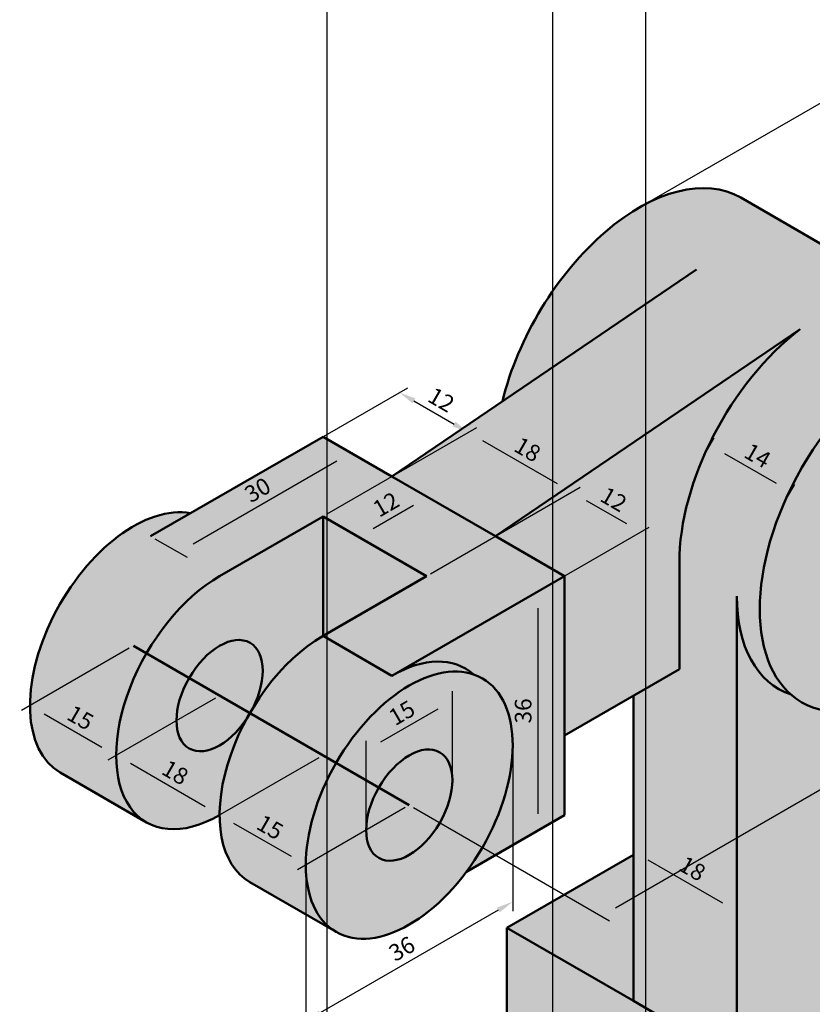
# Model space of a CAD drawing. Units: millimetres. Extents: x 1466 to 1886, y 5011 to 5605.
# Tile 3 of 4: x 1677 to 1796, y 5146 to 5295. Entities that reach past the tile are written whole.
import ezdxf

# ---------------------------------------------------------------- set-up
doc = ezdxf.new("R2010")
doc.units = ezdxf.units.MM
for name, color, linetype, lineweight in [('M-DIMS', 2, 'Continuous', 25), ('M-HATC', 252, 'Continuous', 18), ('M-OUTL', 7, 'Continuous', 50)]:
    doc.layers.add(name, color=color, linetype=linetype, lineweight=lineweight)
doc.styles.get("Standard").update_dxf_attribs({"font": 'arial.ttf'})
doc.dimstyles.new('ISO-25', dxfattribs={"dimtxt": 2.5, "dimasz": 2.5, "dimexe": 1.25, "dimexo": 0.625, "dimtad": 1, "dimtxsty": 'Standard', "dimcen": 2.5, "dimadec": 0, "dimazin": 0, "dimtfac": 1, "dimtmove": 0, "dimatfit": 3, "dimfxl": 1, "dimarcsym": 0})

# ---------------------------------------------------------------- blocks, each defined once
blk = doc.blocks.new('*D1')
at = {"layer": 'Defpoints', "color": 0, "transparency": 16777216}
for p in [(1828.098835256636, 5162.955036981139), (1834.164568784784, 5159.452984095829), (1784.797565067414, 5137.955036981139)]:
    blk.add_point(p, dxfattribs=at)
at = {"layer": 'M-DIMS', "color": 0, "lineweight": -2, "transparency": 16777216}
for p, q in [((1828.723835256636, 5162.594193062894), (1835.414568784784, 5158.731296259342)), ((1793.028362105023, 5135.702984095829), (1831.999505275323, 5158.202984095829)), ((1785.422565067414, 5137.594193062894), (1792.113298595562, 5133.731296259342))]:
    blk.add_line(p, q, dxfattribs=at)
at = {"layer": 'M-DIMS', "color": 0, "transparency": 16777216}
for points in [[(1831.79117194199, 5158.563828014073), (1832.207838608656, 5157.842140177587), (1834.164568784784, 5159.452984095829)], [(1792.82002877169, 5136.063828014073), (1793.236695438357, 5135.342140177587), (1790.863298595562, 5134.45298409583)]]:
    blk.add_solid(points, dxfattribs=at)
at = {"layer": 'M-DIMS', "color": 0, "transparency": 16777216, "insert": (1811.563217455521, 5148.599672917828), "char_height": 2.5, "attachment_point": 5, "rotation": 30.000000000000025}
blk.add_mtext('50', dxfattribs=at)
blk = doc.blocks.new('*D3')
at = {"layer": 'Defpoints', "color": 0, "transparency": 16777216}
for p in [(1770.344853030102, 5217.610759795876), (1738.032193263054, 5210.955036981139), (1748.424498108467, 5204.955036981139)]:
    blk.add_point(p, dxfattribs=at)
at = {"layer": 'M-DIMS', "color": 0, "lineweight": -2, "transparency": 16777216}
for p, q in [((1738.657193263054, 5211.315880899382), (1761.202548184689, 5224.332447632363)), ((1762.11761169415, 5222.360759795876), (1768.179789520641, 5218.860759795877)), ((1749.049498108467, 5205.315880899382), (1771.594853030102, 5218.332447632363))]:
    blk.add_line(p, q, dxfattribs=at)
at = {"layer": 'M-DIMS', "color": 0, "transparency": 16777216}
for points in [[(1762.325945027483, 5222.72160371412), (1761.909278360817, 5221.999915877631), (1759.952548184689, 5223.610759795876)], [(1768.388122853975, 5219.22160371412), (1767.971456187307, 5218.499915877632), (1770.344853030102, 5217.610759795876)]]:
    blk.add_solid(points, dxfattribs=at)
at = {"layer": 'M-DIMS', "color": 0, "transparency": 16777216, "insert": (1766.088758588296, 5222.238987980856), "char_height": 2.5, "attachment_point": 5, "rotation": 330}
blk.add_mtext('12', dxfattribs=at)
blk = doc.blocks.new('*D4')
at = {"layer": 'Defpoints', "color": 0, "transparency": 16777216}
for p in [(1744.364090916567, 5232.610759795876), (1722.443735994934, 5219.955036981137), (1738.032193263055, 5210.955036981139)]:
    blk.add_point(p, dxfattribs=at)
at = {"layer": 'M-DIMS', "color": 0, "lineweight": -2, "transparency": 16777216}
for p, q in [((1723.068735994934, 5220.315880899381), (1745.614090916567, 5233.332447632363)), ((1757.787484675226, 5224.860759795877), (1746.529154426028, 5231.360759795876)), ((1738.657193263054, 5211.315880899382), (1761.202548184687, 5224.332447632364))]:
    blk.add_line(p, q, dxfattribs=at)
at = {"layer": 'M-DIMS', "color": 0, "transparency": 16777216}
for points in [[(1746.737487759362, 5231.72160371412), (1746.320821092695, 5230.999915877633), (1744.364090916567, 5232.610759795876)], [(1757.99581800856, 5225.221603714119), (1757.579151341893, 5224.499915877633), (1759.952548184688, 5223.610759795876)]]:
    blk.add_solid(points, dxfattribs=at)
at = {"layer": 'M-DIMS', "color": 0, "transparency": 16777216, "insert": (1753.10903578528, 5229.757448617874), "char_height": 2.5, "attachment_point": 5, "rotation": 330.0000000000034}
blk.add_mtext('18', dxfattribs=at)
blk = doc.blocks.new('*D5')
at = {"layer": 'Defpoints', "color": 0, "transparency": 16777216}
for p in [(1744.364090916567, 5232.610759795875), (1712.051431149521, 5225.955036981138), (1722.443735994934, 5219.955036981136)]:
    blk.add_point(p, dxfattribs=at)
at = {"layer": 'M-DIMS', "color": 0, "lineweight": -2, "transparency": 16777216}
for p, q in [((1712.676431149521, 5226.315880899382), (1735.221786071155, 5239.332447632363)), ((1736.136849580615, 5237.360759795875), (1742.199027407106, 5233.860759795874)), ((1723.068735994934, 5220.315880899381), (1745.614090916567, 5233.332447632362))]:
    blk.add_line(p, q, dxfattribs=at)
at = {"layer": 'M-DIMS', "color": 0, "transparency": 16777216}
for points in [[(1736.345182913948, 5237.721603714119), (1735.928516247281, 5236.999915877631), (1733.971786071154, 5238.610759795875)], [(1742.407360740439, 5234.221603714118), (1741.990694073772, 5233.499915877629), (1744.364090916567, 5232.610759795875)]]:
    blk.add_solid(points, dxfattribs=at)
at = {"layer": 'M-DIMS', "color": 0, "transparency": 16777216, "insert": (1740.107996474761, 5237.238987980854), "char_height": 2.5, "attachment_point": 5, "rotation": 329.9999999999946}
blk.add_mtext('12', dxfattribs=at)
blk = doc.blocks.new('*D6')
at = {"layer": 'Defpoints', "color": 0, "transparency": 16777216}
for p in [(1779.859746418598, 5229.119875136286), (1792.895839951523, 5223.699051467532), (1791.98410207158, 5222.119875136286)]:
    blk.add_point(p, dxfattribs=at)
at = {"layer": 'M-DIMS', "color": 0, "lineweight": -2, "transparency": 16777216}
for p, q in [((1780.172246418598, 5229.661141013651), (1781.39648429854, 5231.781583222262)), ((1782.936547808002, 5229.449051467532), (1790.730776442061, 5224.949051467532)), ((1792.29660207158, 5222.661141013651), (1793.520839951523, 5224.781583222262))]:
    blk.add_line(p, q, dxfattribs=at)
at = {"layer": 'M-DIMS', "color": 0, "transparency": 16777216}
for points in [[(1783.144881141335, 5229.809895385776), (1782.728214474668, 5229.088207549288), (1780.77148429854, 5230.699051467532)], [(1790.939109775395, 5225.309895385777), (1790.522443108728, 5224.588207549288), (1792.895839951523, 5223.699051467532)]]:
    blk.add_solid(points, dxfattribs=at)
at = {"layer": 'M-DIMS', "color": 0, "transparency": 16777216, "insert": (1787.773720105932, 5228.827279652513), "char_height": 2.5, "attachment_point": 5, "rotation": 329.99999999999994}
blk.add_mtext('14', dxfattribs=at)
blk = doc.blocks.new('*D7')
at = {"layer": 'Defpoints', "color": 0, "transparency": 16777216}
for p in [(1769.209107799294, 5177.115921383499), (1784.797565067414, 5168.115921383499), (1784.797565067414, 5160.477837964851)]:
    blk.add_point(p, dxfattribs=at)
at = {"layer": 'M-DIMS', "color": 0, "lineweight": -2, "transparency": 16777216}
for p, q in [((1769.209107799293, 5176.394233547013), (1769.209107799294, 5168.034462291878)), ((1771.374171308754, 5168.227837964852), (1782.632501557953, 5161.72783796485)), ((1784.797565067413, 5167.39423354701), (1784.797565067414, 5159.034462291876))]:
    blk.add_line(p, q, dxfattribs=at)
at = {"layer": 'M-DIMS', "color": 0, "transparency": 16777216}
for points in [[(1771.582504642088, 5168.588681883095), (1771.165837975421, 5167.866994046608), (1769.209107799294, 5169.477837964851)], [(1782.840834891286, 5162.088681883094), (1782.424168224619, 5161.366994046607), (1784.797565067414, 5160.477837964851)]]:
    blk.add_solid(points, dxfattribs=at)
at = {"layer": 'M-DIMS', "color": 0, "transparency": 16777216, "insert": (1777.954052668006, 5166.624526786849), "char_height": 2.5, "attachment_point": 5, "rotation": 329.99999999999767}
blk.add_mtext('18', dxfattribs=at)
blk = doc.blocks.new('*D8')
at = {"layer": 'Defpoints', "color": 0, "transparency": 16777216}
for p in [(1740.630269474408, 5221.45503698114), (1727.82787069774, 5216.84650536112), (1730.237964628994, 5215.455036981139)]:
    blk.add_point(p, dxfattribs=at)
at = {"layer": 'M-DIMS', "color": 0, "lineweight": -2, "transparency": 16777216}
for p, q in [((1740.005269474408, 5221.815880899383), (1736.970175543155, 5223.568193197609)), ((1736.055112033694, 5221.596505361122), (1729.992934207201, 5218.096505361121)), ((1729.612964628995, 5215.815880899381), (1726.57787069774, 5217.568193197607))]:
    blk.add_line(p, q, dxfattribs=at)
at = {"layer": 'M-DIMS', "color": 0, "transparency": 16777216}
for points in [[(1735.84677870036, 5221.957349279364), (1736.263445367027, 5221.235661442877), (1738.220175543155, 5222.846505361122)], [(1729.784600873868, 5218.457349279363), (1730.201267540534, 5217.735661442877), (1727.82787069774, 5216.84650536112)]]:
    blk.add_solid(points, dxfattribs=at)
at = {"layer": 'M-DIMS', "color": 0, "transparency": 16777216, "insert": (1732.083965139547, 5221.474733546102), "char_height": 2.5, "attachment_point": 5, "rotation": 29.99999999999947}
blk.add_mtext('12', dxfattribs=at)
blk = doc.blocks.new('*D9')
at = {"layer": 'Defpoints', "color": 0, "transparency": 16777216}
for p in [(1722.443735994935, 5231.955036981139), (1696.462973881402, 5216.955036981139), (1700.698632448882, 5214.509578367006)]:
    blk.add_point(p, dxfattribs=at)
at = {"layer": 'M-DIMS', "color": 0, "lineweight": -2, "transparency": 16777216}
for p, q in [((1723.068735994934, 5231.594193062895), (1727.929394562414, 5228.787890530519)), ((1724.514331052953, 5228.259578367006), (1702.863695958343, 5215.759578367006)), ((1697.087973881401, 5216.594193062896), (1701.948632448881, 5213.787890530518))]:
    blk.add_line(p, q, dxfattribs=at)
at = {"layer": 'M-DIMS', "color": 0, "transparency": 16777216}
for points in [[(1724.30599771962, 5228.620422285248), (1724.722664386287, 5227.898734448762), (1726.679394562414, 5229.509578367006)], [(1702.655362625009, 5216.12042228525), (1703.072029291676, 5215.398734448762), (1700.698632448882, 5214.509578367006)]]:
    blk.add_solid(points, dxfattribs=at)
at = {"layer": 'M-DIMS', "color": 0, "transparency": 16777216, "insert": (1712.737870940846, 5223.657005614485), "char_height": 2.5, "attachment_point": 5, "rotation": 29.999999999999872}
blk.add_mtext('30', dxfattribs=at)
blk = doc.blocks.new('*D10')
at = {"layer": 'Defpoints', "color": 0, "transparency": 16777216}
for p in [(1758.816802953882, 5210.955036981141), (1758.816802953882, 5174.95503698114), (1754.826481627799, 5172.651223889373)]:
    blk.add_point(p, dxfattribs=at)
at = {"layer": 'M-DIMS', "color": 0, "lineweight": -2, "transparency": 16777216}
for p, q in [((1758.191802953882, 5210.594193062897), (1753.576481627799, 5207.929536052886)), ((1754.826481627799, 5206.151223889373), (1754.826481627799, 5175.151223889373)), ((1758.191802953882, 5174.594193062898), (1753.576481627799, 5171.929536052886))]:
    blk.add_line(p, q, dxfattribs=at)
at = {"layer": 'M-DIMS', "color": 0, "transparency": 16777216}
for points in [[(1754.409814961132, 5206.151223889373), (1755.243148294466, 5206.151223889373), (1754.826481627799, 5208.651223889373)], [(1754.409814961132, 5175.151223889373), (1755.243148294466, 5175.151223889373), (1754.826481627799, 5172.651223889373)]]:
    blk.add_solid(points, dxfattribs=at)
at = {"layer": 'M-DIMS', "color": 0, "transparency": 16777216, "insert": (1752.924196498195, 5190.651223889371), "char_height": 2.5, "attachment_point": 5, "rotation": 90}
blk.add_mtext('36', dxfattribs=at)
blk = doc.blocks.new('*D11')
at = {"layer": 'Defpoints', "color": 0, "transparency": 16777216}
for p in [(1751.022574319821, 5185.455036981139), (1719.845659783581, 5167.455036981138), (1719.845659783581, 5143.908828507063)]:
    blk.add_point(p, dxfattribs=at)
at = {"layer": 'M-DIMS', "color": 0, "lineweight": -2, "transparency": 16777216}
for p, q in [((1751.022574319821, 5184.733349144652), (1751.022574319821, 5160.465452834088)), ((1719.845659783581, 5166.733349144652), (1719.845659783581, 5142.465452834088)), ((1748.85751081036, 5160.658828507063), (1722.010723293042, 5145.158828507063))]:
    blk.add_line(p, q, dxfattribs=at)
at = {"layer": 'M-DIMS', "color": 0, "transparency": 16777216}
for points in [[(1748.649177477027, 5161.019672425307), (1749.065844143693, 5160.297984588819), (1751.022574319821, 5161.908828507063)], [(1721.802389959709, 5145.519672425306), (1722.219056626375, 5144.797984588819), (1719.845659783581, 5143.908828507063)]]:
    blk.add_solid(points, dxfattribs=at)
at = {"layer": 'M-DIMS', "color": 0, "transparency": 16777216, "insert": (1734.482974486899, 5154.556255754542), "char_height": 2.5, "attachment_point": 5, "rotation": 30.00000000000017}
blk.add_mtext('36', dxfattribs=at)
blk = doc.blocks.new('*D12')
at = {"layer": 'Defpoints', "color": 0, "transparency": 16777216}
for p in [(1728.938926523318, 5184.680108528979), (1741.929307580084, 5180.205036981138), (1728.938926523318, 5172.705036981138)]:
    blk.add_point(p, dxfattribs=at)
at = {"layer": 'M-DIMS', "color": 0, "lineweight": -2, "transparency": 16777216}
for p, q in [((1741.929307580084, 5180.926724817625), (1741.929307580084, 5193.623484201953)), ((1739.764244070623, 5190.93010852898), (1731.103990032779, 5185.93010852898)), ((1728.938926523318, 5173.426724817626), (1728.938926523318, 5186.123484201954))]:
    blk.add_line(p, q, dxfattribs=at)
at = {"layer": 'M-DIMS', "color": 0, "transparency": 16777216}
for points in [[(1739.55591073729, 5191.290952447223), (1739.972577403956, 5190.569264610736), (1741.929307580084, 5192.18010852898)], [(1730.895656699446, 5186.290952447223), (1731.312323366112, 5185.569264610736), (1728.938926523318, 5184.680108528979)]]:
    blk.add_solid(points, dxfattribs=at)
at = {"layer": 'M-DIMS', "color": 0, "transparency": 16777216, "insert": (1734.483400817049, 5190.076797350977), "char_height": 2.5, "attachment_point": 5, "rotation": 29.999999999999872}
blk.add_mtext('15', dxfattribs=at)
blk = doc.blocks.new('*D18')
at = {"layer": 'Defpoints', "color": 0, "transparency": 16777216}
for p in [(1693.864897670048, 5200.455036981139), (1706.855278726814, 5192.955036981139), (1691.266821458693, 5183.955036981138)]:
    blk.add_point(p, dxfattribs=at)
at = {"layer": 'M-DIMS', "color": 0, "lineweight": -2, "transparency": 16777216}
for p, q in [((1693.239897670048, 5200.094193062894), (1677.026440401927, 5190.73334914465)), ((1706.230278726814, 5192.594193062895), (1690.016821458694, 5183.23334914465)), ((1680.441503911388, 5190.205036981137), (1689.101757949233, 5185.205036981137))]:
    blk.add_line(p, q, dxfattribs=at)
at = {"layer": 'M-DIMS', "color": 0, "transparency": 16777216}
for points in [[(1680.649837244722, 5190.565880899381), (1680.233170578055, 5189.844193062894), (1678.276440401927, 5191.455036981138)], [(1689.310091282566, 5185.565880899382), (1688.893424615899, 5184.844193062894), (1691.266821458693, 5183.955036981138)]]:
    blk.add_solid(points, dxfattribs=at)
at = {"layer": 'M-DIMS', "color": 0, "transparency": 16777216, "insert": (1685.722347164963, 5189.351725803136), "char_height": 2.5, "attachment_point": 5, "rotation": 329.99999999999966}
blk.add_mtext('15', dxfattribs=at)
blk = doc.blocks.new('*D19')
at = {"layer": 'Defpoints', "color": 0, "transparency": 16777216}
for p in [(1722.443735994935, 5183.955036981138), (1735.434117051701, 5176.455036981138), (1706.855278726813, 5174.955036981137)]:
    blk.add_point(p, dxfattribs=at)
at = {"layer": 'M-DIMS', "color": 0, "lineweight": -2, "transparency": 16777216}
for p, q in [((1721.818735994935, 5183.594193062894), (1705.605278726813, 5174.23334914465)), ((1734.809117051701, 5176.094193062894), (1718.59565978358, 5166.733349144649)), ((1717.680596274119, 5168.705036981136), (1709.020342236275, 5173.705036981136))]:
    blk.add_line(p, q, dxfattribs=at)
at = {"layer": 'M-DIMS', "color": 0, "transparency": 16777216}
for points in [[(1709.228675569608, 5174.065880899379), (1708.812008902941, 5173.344193062892), (1706.855278726813, 5174.955036981137)], [(1717.888929607452, 5169.065880899379), (1717.472262940785, 5168.344193062893), (1719.84565978358, 5167.455036981135)]]:
    blk.add_solid(points, dxfattribs=at)
at = {"layer": 'M-DIMS', "color": 0, "transparency": 16777216, "insert": (1714.301185489849, 5172.851725803135), "char_height": 2.5, "attachment_point": 5, "rotation": 329.99999999999966}
blk.add_mtext('15', dxfattribs=at)
blk = doc.blocks.new('*D20')
at = {"layer": 'Defpoints', "color": 0, "transparency": 16777216}
for p in [(1706.855278726814, 5192.955036981139), (1691.266821458695, 5183.955036981139), (1722.443735994935, 5183.955036981138)]:
    blk.add_point(p, dxfattribs=at)
at = {"layer": 'M-DIMS', "color": 0, "lineweight": -2, "transparency": 16777216}
for p, q in [((1706.230278726815, 5192.594193062895), (1690.016821458694, 5183.23334914465)), ((1704.690215217354, 5176.205036981137), (1693.431884968156, 5182.705036981139)), ((1721.818735994935, 5183.594193062894), (1705.605278726815, 5174.233349144651))]:
    blk.add_line(p, q, dxfattribs=at)
at = {"layer": 'M-DIMS', "color": 0, "transparency": 16777216}
for points in [[(1693.640218301489, 5183.065880899381), (1693.223551634822, 5182.344193062895), (1691.266821458695, 5183.955036981139)], [(1704.898548550688, 5176.565880899381), (1704.481881884021, 5175.844193062893), (1706.855278726815, 5174.955036981138)]]:
    blk.add_solid(points, dxfattribs=at)
at = {"layer": 'M-DIMS', "color": 0, "transparency": 16777216, "insert": (1700.011766327407, 5181.101725803135), "char_height": 2.5, "attachment_point": 5, "rotation": 330.0000000000005}
blk.add_mtext('18', dxfattribs=at)
blk = doc.blocks.new('*D24')
at = {"layer": 'Defpoints', "color": 0, "transparency": 16777216}
for p in [(1809.046276373379, 5218.955036981139), (1837.969099370778, 5202.256437337866), (1735.434117051702, 5176.455036981138)]:
    blk.add_point(p, dxfattribs=at)
at = {"layer": 'M-DIMS', "color": 0, "lineweight": -2, "transparency": 16777216}
for p, q in [((1809.671276373379, 5218.594193062894), (1839.219099370778, 5201.534749501379)), ((1766.522003558562, 5161.006437337866), (1835.804035861317, 5201.006437337866)), ((1736.059117051701, 5176.094193062894), (1765.606940049101, 5159.03474950138))]:
    blk.add_line(p, q, dxfattribs=at)
at = {"layer": 'M-DIMS', "color": 0, "transparency": 16777216}
for points in [[(1835.595702527983, 5201.367281256109), (1836.01236919465, 5200.645593419623), (1837.969099370778, 5202.256437337866)], [(1766.313670225229, 5161.367281256109), (1766.730336891895, 5160.645593419623), (1764.356940049101, 5159.756437337867)]]:
    blk.add_solid(points, dxfattribs=at)
at = {"layer": 'M-DIMS', "color": 0, "transparency": 16777216, "insert": (1800.212303475287, 5182.653126159864), "char_height": 2.5, "attachment_point": 5, "rotation": 29.99999999999997}
blk.add_mtext('85', dxfattribs=at)
blk = doc.blocks.new('*D25')
at = {"layer": 'Defpoints', "color": 0, "transparency": 16777216}
for p in [(1800.844478091805, 5284.219726535433), (1770.07513320308, 5266.455036981138), (1809.912301777163, 5243.45503698114)]:
    blk.add_point(p, dxfattribs=at)
at = {"layer": 'M-DIMS', "color": 0, "lineweight": -2, "transparency": 16777216}
for p, q in [((1770.70013320308, 5266.815880899383), (1802.094478091805, 5284.941414371921)), ((1838.516583156427, 5262.469726535435), (1803.009541601266, 5282.969726535434)), ((1810.537301777163, 5243.815880899384), (1841.931646665887, 5261.941414371922))]:
    blk.add_line(p, q, dxfattribs=at)
at = {"layer": 'M-DIMS', "color": 0, "transparency": 16777216}
for points in [[(1803.2178749346, 5283.330570453678), (1802.801208267933, 5282.608882617189), (1800.844478091805, 5284.219726535433)], [(1838.72491648976, 5262.830570453679), (1838.308249823093, 5262.108882617191), (1840.681646665888, 5261.219726535435)]]:
    blk.add_solid(points, dxfattribs=at)
at = {"layer": 'M-DIMS', "color": 0, "transparency": 16777216, "insert": (1821.713778613498, 5274.366415357433), "char_height": 2.5, "attachment_point": 5, "rotation": 330.0000000000001}
blk.add_mtext('46', dxfattribs=at)
blk = doc.blocks.new('*D57')
at = {"layer": 'Defpoints', "color": 0, "transparency": 16777216}
for p in [(1723.014464, 5426.716336000001), (1757.014464, 5426.716336000001), (1757.014464, 5011.829342)]:
    blk.add_point(p, dxfattribs=at)
at = {"layer": 'M-DIMS', "color": 0, "lineweight": -2, "transparency": 16777216}
for p, q in [((1723.014464, 5426.091336), (1723.014464, 5010.579341999999)), ((1757.014464, 5426.091336), (1757.014464, 5010.579341999999)), ((1725.514464, 5011.829342), (1754.514464, 5011.829342))]:
    blk.add_line(p, q, dxfattribs=at)
at = {"layer": 'M-DIMS', "color": 0, "transparency": 16777216}
for points in [[(1725.514464, 5012.246008666667), (1725.514464, 5011.412675333333), (1723.014464, 5011.829342)], [(1754.514464, 5012.246008666667), (1754.514464, 5011.412675333333), (1757.014464, 5011.829342)]]:
    blk.add_solid(points, dxfattribs=at)
at = {"layer": 'M-DIMS', "color": 0, "transparency": 16777216, "insert": (1740.014464, 5013.731627129605), "char_height": 2.5, "attachment_point": 5}
blk.add_mtext('34', dxfattribs=at)
blk = doc.blocks.new('*D58')
at = {"layer": 'Defpoints', "color": 0, "transparency": 16777216}
for p in [(1757.014464, 5426.716336000001), (1771.014464, 5426.716336000001), (1771.014464, 5011.829342)]:
    blk.add_point(p, dxfattribs=at)
at = {"layer": 'M-DIMS', "color": 0, "lineweight": -2, "transparency": 16777216}
for p, q in [((1757.014464, 5426.091336), (1757.014464, 5010.579341999999)), ((1771.014464, 5426.091336), (1771.014464, 5010.579341999999)), ((1759.514464, 5011.829342), (1768.514464, 5011.829342))]:
    blk.add_line(p, q, dxfattribs=at)
at = {"layer": 'M-DIMS', "color": 0, "transparency": 16777216}
for points in [[(1759.514464, 5012.246008666667), (1759.514464, 5011.412675333333), (1757.014464, 5011.829342)], [(1768.514464, 5012.246008666667), (1768.514464, 5011.412675333333), (1771.014464, 5011.829342)]]:
    blk.add_solid(points, dxfattribs=at)
at = {"layer": 'M-DIMS', "color": 0, "transparency": 16777216, "insert": (1764.014464, 5013.709457961801), "char_height": 2.5, "attachment_point": 5}
blk.add_mtext('14', dxfattribs=at)

msp = doc.modelspace()

# ---------------------------------------------------------------- hatches: boundary and pattern name
at = {"layer": 'M-HATC'}
h = msp.add_hatch(color=256, dxfattribs=at)
h.dxf.hatch_style = 1
edge = h.paths.add_edge_path()
edge.add_line((1722.443735994935, 5219.955036981139), (1738.032193263055, 5210.955036981139))
edge.add_line((1738.032193263055, 5210.955036981139), (1722.443735994935, 5201.955036981138))
edge.add_line((1722.443735994935, 5201.955036981138), (1732.836040840348, 5195.955036981139))
edge.add_line((1732.836040840348, 5195.955036981139), (1758.816802953881, 5210.955036981139))
edge.add_line((1758.816802953881, 5210.955036981139), (1748.424498108468, 5216.955036981139))
edge.add_line((1748.424498108468, 5216.955036981139), (1732.836040840348, 5225.955036981138))
edge.add_line((1732.836040840348, 5225.955036981138), (1722.443735994935, 5231.955036981139))
edge.add_line((1722.443735994935, 5231.955036981139), (1712.051431149521, 5225.955036981138))
edge.add_line((1712.051431149521, 5225.955036981138), (1702.481741639855, 5220.429974166671))
edge.add_ellipse((1693.864897670048, 5200.455036981139), major_axis=(-11.02270384252446, -19.0918830920367), ratio=0.5773502691896324, start_angle=186.6654644117269, end_angle=360)
edge.add_line((1682.842193827524, 5181.363153889102), (1695.83257488429, 5173.863153889102))
edge.add_ellipse((1706.855278726814, 5192.955036981139), major_axis=(-11.02270384252446, -19.09188309203669), ratio=0.5773502691896325, start_angle=270, end_angle=359.9999999999998, ccw=False)
edge.add_ellipse((1706.855278726814, 5192.955036981139), major_axis=(-11.02270384252446, -19.09188309203669), ratio=0.5773502691896325, start_angle=210.0000000000012, end_angle=270, ccw=False)
edge.add_line((1706.855278726813, 5210.955036981138), (1722.443735994935, 5219.955036981139))
edge = h.paths.add_edge_path(flags=17)
edge.add_ellipse((1735.434117051701, 5176.455036981138), major_axis=(-11.02270384252446, -19.0918830920367), ratio=0.5773502691896324, start_angle=183.919715644874, end_angle=270, ccw=False)
edge.add_ellipse((1732.836040840348, 5177.955036981138), major_axis=(-11.02270384252446, -19.0918830920367), ratio=0.5773502691896323, start_angle=176.0802843551266, end_angle=210.0000000000004)
edge.add_line((1732.836040840348, 5195.955036981139), (1722.443735994935, 5201.955036981138))
edge.add_ellipse((1722.443735994935, 5183.955036981139), major_axis=(-11.02270384252446, -19.0918830920367), ratio=0.5773502691896323, start_angle=210.0000000000004, end_angle=266.235889459397)
edge.add_ellipse((1706.855278726814, 5192.955036981139), major_axis=(-4.592793267718468, -7.954951288348655), ratio=0.5773502691896232, start_angle=90, end_angle=99.00326933995552, ccw=False)
edge.add_line((1711.448071994533, 5190.303386551689), (1724.411413209177, 5182.818998011818))
edge = h.paths.add_edge_path()
edge.add_line((1724.411413209177, 5182.818998011818), (1711.448071994533, 5190.303386551689))
edge.add_ellipse((1706.855278726814, 5192.955036981139), major_axis=(-4.592793267718468, -7.954951288348655), ratio=0.5773502691896232, start_angle=80.9967306600526, end_angle=90, ccw=False)
edge.add_ellipse((1722.443735994935, 5183.955036981139), major_axis=(-11.02270384252446, -19.0918830920367), ratio=0.5773502691896323, start_angle=273.764110540599, end_angle=329.9999999999981)
edge.add_ellipse((1722.443735994935, 5183.955036981139), major_axis=(-11.02270384252446, -19.0918830920367), ratio=0.5773502691896323, start_angle=329.9999999999981, end_angle=360)
edge.add_line((1711.42103215241, 5164.863153889102), (1724.411413209177, 5157.363153889102))
edge.add_ellipse((1735.434117051701, 5176.455036981138), major_axis=(-11.02270384252446, -19.0918830920367), ratio=0.5773502691896324, start_angle=270, end_angle=360, ccw=False)
edge = h.paths.add_edge_path(flags=17)
edge.add_line((1758.816802953881, 5210.955036981139), (1732.836040840348, 5195.955036981139))
edge.add_ellipse((1732.836040840348, 5177.955036981138), major_axis=(-11.02270384252446, -19.0918830920367), ratio=0.5773502691896323, start_angle=176.0802843551266, end_angle=210.0000000000005, ccw=False)
edge.add_ellipse((1735.434117051701, 5176.455036981138), major_axis=(-11.02270384252446, -19.0918830920367), ratio=0.5773502691896324, start_angle=70.6800531201103, end_angle=183.919715644874, ccw=False)
edge.add_line((1744.050961021509, 5166.429974166671), (1758.816802953881, 5174.955036981138))
edge.add_line((1758.816802953881, 5174.955036981138), (1758.816802953881, 5210.955036981139))
edge = h.paths.add_edge_path(flags=17)
edge.add_ellipse((1797.78794612418, 5225.455036981139), major_axis=(-15.30931089239438, -26.5165042944958), ratio=0.5773502691896226, start_angle=218.6849191088683, end_angle=329.99999999999915, ccw=False)
edge.add_line((1794.323844509042, 5248.132962339644), (1748.424498108468, 5216.955036981139))
edge.add_line((1748.424498108468, 5216.955036981139), (1758.816802953881, 5210.955036981139))
edge.add_line((1758.816802953881, 5210.955036981139), (1758.816802953881, 5186.955036981139))
edge.add_line((1758.816802953881, 5186.955036981139), (1776.13731102957, 5196.955036981139))
edge.add_line((1776.13731102957, 5196.955036981139), (1776.13731102957, 5212.955036981139))
edge = h.paths.add_edge_path()
edge.add_ellipse((1797.78794612418, 5225.455036981139), major_axis=(-15.30931089239438, -26.5165042944958), ratio=0.5773502691896226, start_angle=218.6849191088682, end_angle=329.9999999999991)
edge.add_line((1776.13731102957, 5212.955036981139), (1776.13731102957, 5196.955036981139))
edge.add_line((1776.13731102957, 5196.955036981139), (1769.209107799294, 5192.955036981139))
edge.add_line((1769.209107799294, 5192.955036981139), (1769.209107799294, 5146.955036981139))
edge.add_line((1769.209107799294, 5146.955036981139), (1784.797565067414, 5137.955036981139))
edge.add_line((1784.797565067414, 5137.955036981139), (1784.797565067414, 5155.95503698114))
edge.add_line((1784.797565067414, 5155.95503698114), (1784.797565067414, 5207.955036981145))
edge.add_ellipse((1806.448200162025, 5220.455036981139), major_axis=(-15.30931089239438, -26.5165042944958), ratio=0.5773502691896227, start_angle=329.9999999999989, end_angle=363.7613167964908)
edge.add_ellipse((1809.912301777163, 5218.455036981139), major_axis=(-15.30931089239438, -26.5165042944958), ratio=0.5773502691896226, start_angle=179.9999999999992, end_angle=356.23868320351306, ccw=False)
edge.add_line((1825.221612669557, 5244.971541275634), (1785.384444095473, 5267.971541275635))
edge.add_ellipse((1770.075133203079, 5241.455036981139), major_axis=(-15.30931089239438, -26.5165042944958), ratio=0.5773502691896226, start_angle=540, end_angle=311.5164128123438)
edge.add_line((1749.475859885243, 5237.257922029503), (1732.836040840348, 5225.955036981138))
edge.add_line((1732.836040840348, 5225.955036981138), (1748.424498108468, 5216.955036981139))
edge.add_line((1748.424498108468, 5216.955036981139), (1794.323844509042, 5248.132962339644))
edge = h.paths.add_edge_path()
edge.add_line((1828.098835256636, 5207.955036981139), (1825.221612669557, 5209.616202216307))
edge.add_ellipse((1809.912301777163, 5218.455036981139), major_axis=(-15.30931089239438, -26.5165042944958), ratio=0.5773502691896226, start_angle=356.23868320351306, end_angle=449.99999999999966, ccw=False)
edge.add_ellipse((1806.448200162025, 5220.455036981139), major_axis=(-15.30931089239438, -26.5165042944958), ratio=0.5773502691896227, start_angle=329.99999999999886, end_angle=363.76131679649075, ccw=False)
edge.add_line((1784.797565067414, 5207.955036981145), (1784.797565067414, 5155.95503698114))
edge.add_line((1784.797565067414, 5155.95503698114), (1784.797565067414, 5137.955036981139))
edge.add_line((1784.797565067414, 5137.955036981139), (1828.098835256636, 5162.955036981139))
edge.add_line((1828.098835256636, 5162.955036981139), (1828.098835256636, 5207.955036981139))
edge = h.paths.add_edge_path()
edge.add_ellipse((1809.912301777163, 5218.455036981139), major_axis=(-15.30931089239438, -26.5165042944958), ratio=0.5773502691896226, start_angle=89.99999999999972, end_angle=110.43480323036249, ccw=False)
edge.add_line((1825.221612669557, 5209.616202216307), (1828.098835256636, 5207.955036981139))
edge.add_line((1828.098835256636, 5207.955036981139), (1828.098835256636, 5215.390377014889))
h.paths.add_polyline_path([(1769.209107799294, 5168.955036981138), (1750.156548916036, 5157.955036981139), (1769.209107799294, 5146.955036981139)], flags=17)
h.paths.add_polyline_path([(1847.151394139893, 5151.955036981139), (1828.098835256636, 5162.955036981139), (1784.797565067414, 5137.955036981139), (1803.850123950671, 5126.955036981138)])
edge = h.paths.add_edge_path()
edge.add_ellipse((1825.500759045282, 5099.455036981138), major_axis=(-17.14642819948207, -29.69848480983509), ratio=0.577350269189623, start_angle=176.6451013603207, end_angle=299.71017051362753, ccw=False)
edge.add_ellipse((1828.96486066042, 5097.455036981139), major_axis=(-17.14642819948207, -29.69848480983509), ratio=0.577350269189623, start_angle=177.9252840891673, end_angle=183.3548986396804, ccw=False)
edge.add_line((1847.151394139893, 5126.47529615859), (1847.151394139893, 5151.955036981139))
edge.add_line((1847.151394139893, 5151.955036981139), (1804.3764033923, 5127.258884558432))
edge.add_ellipse((1813.3764033923, 5106.455036981138), major_axis=(-17.14642819948207, -29.69848480983509), ratio=0.577350269189623, start_angle=233.3939017938641, end_angle=235.1951901217888)
edge.add_line((1803.850123950671, 5126.703823360306), (1803.850123950671, 5099.564557194057))
edge = h.paths.add_edge_path()
edge.add_ellipse((1828.96486066042, 5097.455036981139), major_axis=(-17.14642819948207, -29.69848480983509), ratio=0.577350269189623, start_angle=183.3548986396804, end_angle=360, ccw=False)
edge.add_ellipse((1825.500759045282, 5099.455036981138), major_axis=(-17.14642819948207, -29.69848480983509), ratio=0.577350269189623, start_angle=176.6451013603206, end_angle=299.7101705136275)
edge.add_line((1803.850123950671, 5099.564557194057), (1803.850123950671, 5126.703823360306))
edge.add_line((1803.850123950671, 5126.703823360306), (1803.850123950671, 5126.955036981138))
edge.add_line((1803.850123950671, 5126.955036981138), (1784.797565067414, 5137.955036981139))
edge.add_line((1784.797565067414, 5137.955036981139), (1769.209107799294, 5146.955036981139))
edge.add_line((1769.209107799294, 5146.955036981139), (1750.156548916036, 5157.955036981139))
edge.add_line((1750.156548916036, 5157.955036981139), (1750.156548916036, 5139.867928007788))
edge.add_ellipse((1769.165624306577, 5133.458728431643), major_axis=(-17.14642819948207, -29.69848480983509), ratio=0.577350269189623, start_angle=281.3676816797435, end_angle=360)
edge.add_line((1752.019196107095, 5103.760243621808), (1765.421555363387, 5094.680341464254))
edge.add_ellipse((1783.931539663629, 5123.455036981138), major_axis=(-17.14642819948207, -29.69848480983509), ratio=0.577350269189623, start_angle=299.7101705136324, end_angle=357.2479180547133, ccw=False)
edge.add_line((1762.280904569018, 5123.564557194055), (1762.280904569018, 5138.955036981139))
edge.add_line((1762.280904569018, 5138.955036981139), (1784.797565067414, 5125.955036981139))
edge.add_line((1784.797565067414, 5125.955036981139), (1791.725768297689, 5121.955036981138))
edge.add_line((1791.725768297689, 5121.955036981138), (1791.725768297689, 5106.564557194055))
edge.add_ellipse((1813.3764033923, 5106.455036981138), major_axis=(-17.14642819948207, -29.69848480983509), ratio=0.577350269189623, start_angle=299.7101705136277, end_angle=315.9583021122638)
edge.add_ellipse((1813.3764033923, 5106.455036981138), major_axis=(-17.14642819948207, -29.69848480983509), ratio=0.577350269189623, start_angle=315.9583021122638, end_angle=360)
edge.add_line((1796.229975192818, 5076.756552171303), (1811.818432460938, 5067.756552171303))
h = msp.add_hatch(color=256, dxfattribs=at)
h.dxf.hatch_style = 1
edge = h.paths.add_edge_path()
edge.add_ellipse((1809.912301777163, 5218.455036981139), major_axis=(-7.654655446197786, -13.25825214724756), ratio=0.5773502691896373, start_angle=90, end_angle=360, ccw=False)
edge.add_line((1817.56695722336, 5214.035619598722), (1825.221612669557, 5209.616202216307))
edge.add_ellipse((1809.912301777163, 5218.455036981139), major_axis=(-15.30931089239438, -26.5165042944958), ratio=0.5773502691896226, start_angle=89.99999999999962, end_angle=110.4348032303624)
edge.add_ellipse((1809.912301777163, 5218.455036981139), major_axis=(-15.30931089239438, -26.5165042944958), ratio=0.5773502691896226, start_angle=110.4348032303624, end_angle=179.9999999999991)
edge.add_ellipse((1809.912301777163, 5218.455036981139), major_axis=(-15.30931089239438, -26.5165042944958), ratio=0.5773502691896226, start_angle=179.9999999999991, end_angle=356.2386832035131)
edge.add_ellipse((1809.912301777163, 5218.455036981139), major_axis=(-15.30931089239438, -26.5165042944958), ratio=0.5773502691896226, start_angle=356.2386832035131, end_angle=449.9999999999996)
edge.add_line((1825.221612669557, 5209.616202216307), (1817.56695722336, 5214.035619598722))
edge.add_ellipse((1809.912301777163, 5218.455036981139), major_axis=(-7.654655446197786, -13.25825214724756), ratio=0.5773502691896373, start_angle=0, end_angle=90, ccw=False)
edge = h.paths.add_edge_path()
edge.add_ellipse((1735.434117051701, 5176.455036981138), major_axis=(-11.02270384252446, -19.0918830920367), ratio=0.5773502691896324, start_angle=70.68005312011024, end_angle=183.9197156448739)
edge.add_ellipse((1735.434117051701, 5176.455036981138), major_axis=(-11.02270384252446, -19.0918830920367), ratio=0.5773502691896324, start_angle=183.9197156448739, end_angle=270)
edge.add_line((1724.411413209177, 5182.818998011818), (1730.841323783983, 5179.106687410587))
edge.add_ellipse((1735.434117051701, 5176.455036981138), major_axis=(-4.592793267718468, -7.954951288348655), ratio=0.5773502691896234, start_angle=0, end_angle=270, ccw=False)
edge.add_ellipse((1735.434117051701, 5176.455036981138), major_axis=(-4.592793267718468, -7.954951288348655), ratio=0.5773502691896234, start_angle=270, end_angle=360, ccw=False)
edge.add_line((1730.841323783983, 5179.106687410587), (1724.411413209177, 5182.818998011818))
edge.add_ellipse((1735.434117051701, 5176.455036981138), major_axis=(-11.02270384252446, -19.0918830920367), ratio=0.5773502691896324, start_angle=270, end_angle=360)
edge.add_ellipse((1735.434117051701, 5176.455036981138), major_axis=(-11.02270384252446, -19.0918830920367), ratio=0.5773502691896324, start_angle=0, end_angle=70.68005312011029)
edge = h.paths.add_edge_path()
edge.add_line((1722.443735994935, 5219.955036981139), (1706.855278726813, 5210.955036981138))
edge.add_ellipse((1706.855278726814, 5192.955036981139), major_axis=(-11.02270384252446, -19.09188309203669), ratio=0.5773502691896325, start_angle=210.0000000000012, end_angle=270)
edge.add_line((1695.83257488429, 5199.318998011818), (1702.262485459096, 5195.606687410588))
edge.add_ellipse((1706.855278726814, 5192.955036981139), major_axis=(-4.592793267718468, -7.954951288348655), ratio=0.5773502691896232, start_angle=99.00326933995552, end_angle=270, ccw=False)
edge.add_ellipse((1722.443735994935, 5183.955036981139), major_axis=(-11.02270384252446, -19.0918830920367), ratio=0.5773502691896323, start_angle=210.0000000000005, end_angle=266.2358894593971, ccw=False)
edge.add_line((1722.443735994935, 5201.955036981138), (1722.443735994935, 5219.955036981139))
edge = h.paths.add_edge_path()
edge.add_ellipse((1722.443735994935, 5183.955036981139), major_axis=(-11.02270384252446, -19.0918830920367), ratio=0.5773502691896323, start_angle=273.76411054059906, end_angle=329.9999999999982, ccw=False)
edge.add_ellipse((1706.855278726814, 5192.955036981139), major_axis=(-4.592793267718468, -7.954951288348655), ratio=0.5773502691896232, start_angle=270, end_angle=440.9967306600526, ccw=False)
edge.add_line((1702.262485459096, 5195.606687410588), (1695.83257488429, 5199.318998011818))
edge.add_ellipse((1706.855278726814, 5192.955036981139), major_axis=(-11.02270384252446, -19.09188309203669), ratio=0.5773502691896325, start_angle=270, end_angle=359.9999999999997)
edge.add_ellipse((1706.855278726814, 5192.955036981139), major_axis=(-11.02270384252446, -19.09188309203669), ratio=0.5773502691896325, start_angle=359.9999999999997, end_angle=390.0000000000012)
edge = h.paths.add_edge_path()
edge.add_ellipse((1828.96486066042, 5097.455036981139), major_axis=(-17.14642819948207, -29.69848480983509), ratio=0.577350269189623, start_angle=0, end_angle=177.9252840891672)
edge.add_ellipse((1828.96486066042, 5097.455036981139), major_axis=(-17.14642819948207, -29.69848480983509), ratio=0.577350269189623, start_angle=177.9252840891672, end_angle=183.3548986396804)
edge.add_ellipse((1828.96486066042, 5097.455036981139), major_axis=(-17.14642819948207, -29.69848480983509), ratio=0.577350269189623, start_angle=183.3548986396804, end_angle=360)
edge = h.paths.add_edge_path(flags=16)
edge.add_ellipse((1828.96486066042, 5097.455036981139), major_axis=(-9.79795897113284, -16.97056274847708), ratio=0.5773502691896234, start_angle=217.1598249325803, end_angle=322.84017506741907, ccw=False)
edge.add_ellipse((1828.96486066042, 5097.455036981139), major_axis=(-9.79795897113284, -16.97056274847708), ratio=0.5773502691896234, start_angle=322.84017506741907, end_angle=577.1598249325802, ccw=False)
edge = h.paths.add_edge_path()
edge.add_line((1791.725768297689, 5106.564557194055), (1791.725768297689, 5114.726280425816))
edge.add_ellipse((1783.931539663629, 5123.455036981138), major_axis=(-9.797958971132836, -16.97056274847707), ratio=0.5773502691896235, start_angle=322.84017506742066, end_angle=431.7628416390562, ccw=False)
edge.add_ellipse((1783.931539663629, 5123.455036981138), major_axis=(-9.797958971132836, -16.97056274847707), ratio=0.5773502691896235, start_angle=256.9555772654587, end_angle=322.84017506742066, ccw=False)
edge.add_line((1775.519115469529, 5131.31195235414), (1762.280904569018, 5138.955036981139))
edge.add_line((1762.280904569018, 5138.955036981139), (1762.280904569018, 5123.564557194055))
edge.add_ellipse((1783.931539663629, 5123.455036981138), major_axis=(-17.14642819948207, -29.69848480983509), ratio=0.577350269189623, start_angle=299.7101705136324, end_angle=357.2479180547133)
edge.add_line((1765.421555363387, 5094.680341464254), (1766.785111464145, 5093.756552171305))
edge.add_ellipse((1783.931539663629, 5123.455036981138), major_axis=(-17.14642819948207, -29.69848480983509), ratio=0.577350269189623, start_angle=359.9999999999943, end_angle=404.0416978877337)
edge.add_ellipse((1813.3764033923, 5106.455036981138), major_axis=(-17.14642819948207, -29.69848480983509), ratio=0.577350269189623, start_angle=299.71017051362776, end_angle=315.95830211226377, ccw=False)
h = msp.add_hatch(color=256, dxfattribs=at)
h.dxf.hatch_style = 1
edge = h.paths.add_edge_path()
edge.add_ellipse((1735.434117051701, 5176.455036981138), major_axis=(-4.592793267718468, -7.954951288348655), ratio=0.5773502691896234, start_angle=0, end_angle=270)
edge.add_ellipse((1735.434117051701, 5176.455036981138), major_axis=(-4.592793267718468, -7.954951288348655), ratio=0.5773502691896234, start_angle=270, end_angle=360)
edge = h.paths.add_edge_path()
edge.add_ellipse((1809.912301777163, 5218.455036981139), major_axis=(-7.654655446197786, -13.25825214724756), ratio=0.5773502691896373, start_angle=90.00000000000003, end_angle=360)
edge.add_ellipse((1809.912301777163, 5218.455036981139), major_axis=(-7.654655446197786, -13.25825214724756), ratio=0.5773502691896373, start_angle=0, end_angle=90)
edge = h.paths.add_edge_path()
edge.add_ellipse((1706.855278726814, 5192.955036981139), major_axis=(-4.592793267718468, -7.954951288348655), ratio=0.5773502691896232, start_angle=99.00326933995547, end_angle=270)
edge.add_line((1702.262485459096, 5195.606687410588), (1711.42103215241, 5190.318998011818))
edge.add_ellipse((1722.443735994935, 5183.955036981139), major_axis=(-11.02270384252446, -19.0918830920367), ratio=0.5773502691896323, start_angle=266.2358894593971, end_angle=270, ccw=False)
edge = h.paths.add_edge_path()
edge.add_ellipse((1722.443735994935, 5183.955036981139), major_axis=(-11.02270384252446, -19.0918830920367), ratio=0.5773502691896323, start_angle=270, end_angle=273.76411054059906, ccw=False)
edge.add_line((1711.42103215241, 5190.318998011818), (1702.262485459096, 5195.606687410588))
edge.add_ellipse((1706.855278726814, 5192.955036981139), major_axis=(-4.592793267718468, -7.954951288348655), ratio=0.5773502691896232, start_angle=270, end_angle=440.9967306600525)
edge = h.paths.add_edge_path()
edge.add_ellipse((1828.96486066042, 5097.455036981139), major_axis=(-9.79795897113284, -16.97056274847708), ratio=0.5773502691896234, start_angle=322.840175067419, end_angle=217.1598249325803)
edge.add_ellipse((1813.3764033923, 5106.455036981138), major_axis=(-9.797958971132836, -16.97056274847707), ratio=0.5773502691896235, start_angle=397.1598249325802, end_angle=502.8401750674186, ccw=False)
edge = h.paths.add_edge_path()
edge.add_line((1791.725768297689, 5121.955036981138), (1784.797565067414, 5125.955036981139))
edge.add_line((1784.797565067414, 5125.955036981139), (1779.353582800964, 5129.098121608137))
edge.add_ellipse((1768.343082395509, 5132.455036981139), major_axis=(-9.797958971132836, -16.97056274847707), ratio=0.5773502691896235, start_angle=397.1598249325797, end_angle=463.0444227345428, ccw=False)
edge.add_ellipse((1783.931539663629, 5123.455036981138), major_axis=(-9.797958971132836, -16.97056274847707), ratio=0.5773502691896235, start_angle=322.8401750674207, end_angle=431.7628416390561)
edge.add_line((1791.725768297689, 5114.726280425816), (1791.725768297689, 5121.955036981138))
h = msp.add_hatch(color=256, dxfattribs=at)
h.dxf.hatch_style = 1
h.paths.add_polyline_path([(1738.032193263055, 5210.955036981139), (1722.443735994935, 5219.955036981139), (1722.443735994935, 5201.955036981138)])

# ---------------------------------------------------------------- linework, layer by layer
at = {"layer": 'M-OUTL'}
for p, q in [((1825.221612669557, 5244.971541275634), (1785.384444095473, 5267.971541275635)), ((1732.836040840348, 5225.955036981138), (1778.735387240923, 5257.132962339645)), ((1748.424498108468, 5216.955036981139), (1794.323844509043, 5248.132962339645)), ((1712.051431149521, 5225.955036981138), (1722.443735994935, 5231.955036981139)), ((1722.443735994935, 5231.955036981139), (1732.836040840348, 5225.955036981138)), ((1696.462973881401, 5216.955036981139), (1712.051431149521, 5225.955036981138)), ((1732.836040840348, 5225.955036981138), (1748.424498108468, 5216.955036981139)), ((1706.855278726814, 5210.955036981139), (1722.443735994935, 5219.955036981139)), ((1722.443735994935, 5219.955036981139), (1738.032193263055, 5210.955036981139)), ((1722.443735994935, 5219.955036981139), (1722.443735994935, 5201.955036981138)), ((1748.424498108468, 5216.955036981139), (1758.816802953881, 5210.955036981139)), ((1776.13731102957, 5212.955036981139), (1776.13731102957, 5196.955036981139)), ((1738.032193263055, 5210.955036981139), (1722.443735994935, 5201.955036981138)), ((1732.836040840348, 5195.955036981139), (1758.816802953881, 5210.955036981139)), ((1758.816802953881, 5210.955036981139), (1758.816802953881, 5174.955036981138)), ((1784.797565067414, 5155.95503698114), (1784.797565067414, 5207.955036981139)), ((1722.443735994935, 5201.955036981138), (1732.836040840348, 5195.955036981139)), ((1735.434117051701, 5176.455036981138), (1693.864897670048, 5200.455036981139)), ((1758.816802953881, 5186.955036981139), (1776.137311029569, 5196.955036981139)), ((1769.209107799294, 5146.955036981139), (1769.209107799294, 5192.955036981139)), ((1711.448071994533, 5190.303386551689), (1711.42103215241, 5190.318998011818)), ((1695.83257488429, 5173.863153889102), (1682.842193827524, 5181.363153889102)), ((1758.816802953881, 5174.955036981138), (1744.050961021508, 5166.429974166671)), ((1750.156548916036, 5157.955036981139), (1769.209107799294, 5168.955036981138)), ((1724.411413209177, 5157.363153889102), (1711.42103215241, 5164.863153889102)), ((1769.209107799294, 5146.955036981139), (1750.156548916036, 5157.955036981139)), ((1750.156548916036, 5157.955036981139), (1750.156548916036, 5130.564557194056)), ((1784.797565067414, 5137.955036981139), (1784.797565067414, 5155.95503698114)), ((1784.797565067414, 5137.955036981139), (1769.209107799294, 5146.955036981139))]:
    msp.add_line(p, q, dxfattribs=at)
for centre, major_axis, ratio, start_param, end_param in [((1770.075133203079, 5241.455036981139), (-15.30931089239438, -26.5165042944958), 0.5773502691896226, 9.42477796076938, 11.46805550344217), ((1797.78794612418, 5225.455036981139), (-15.30931089239438, -26.5165042944958), 0.5773502691896226, 4.087681469939083, 5.497787143782117), ((1693.864897670048, 5200.455036981139), (-11.02270384252445, -19.09188309203669), 0.5773502691896324, 3.34130527353011, 6.283185307179586), ((1706.855278726814, 5192.955036981139), (-11.02270384252445, -19.09188309203669), 0.5773502691896325, 3.926990816987259, 7.068583470577053), ((1806.448200162025, 5220.455036981139), (-15.30931089239438, -26.5165042944958), 0.5773502691896226, 5.497787143782112, 6.396565152197914), ((1722.443735994935, 5183.955036981139), (-11.02270384252445, -19.09188309203669), 0.5773502691896323, 3.926990816987244, 6.283185307179586), ((1732.836040840348, 5177.955036981138), (-11.02270384252445, -19.09188309203669), 0.5773502691896323, 3.023467000597312, 3.926990816987244)]:
    msp.add_ellipse(centre, major_axis=major_axis, ratio=ratio, start_param=start_param, end_param=end_param, dxfattribs=at)
for centre, major_axis, ratio in [((1809.912301777163, 5218.455036981139), (-15.30931089239438, -26.5165042944958), 0.5773502691896226), ((1706.855278726814, 5192.955036981139), (-4.592793267718467, -7.954951288348654), 0.5773502691896234), ((1735.434117051701, 5176.455036981138), (-11.02270384252445, -19.09188309203669), 0.5773502691896324), ((1735.434117051701, 5176.455036981138), (-4.592793267718467, -7.954951288348654), 0.5773502691896234)]:
    msp.add_ellipse(centre, major_axis=major_axis, ratio=ratio, dxfattribs=at)

# ---------------------------------------------------------------- dimensions: what is measured, and where the dimension line sits
at = {"layer": 'M-DIMS'}
for base, p1, p2, picture, middle in [((1757.014464, 5011.829342), (1723.014464, 5426.716336000001), (1757.014464, 5426.716336000001), '*D57', (1740.014464, 5013.731627129605)), ((1771.014464, 5011.829342), (1757.014464, 5426.716336000001), (1771.014464, 5426.716336000001), '*D58', (1764.014464, 5013.709457961801))]:
    dim = msp.add_linear_dim(base=base, p1=p1, p2=p2, dimstyle='ISO-25', override={"dimdec": 0, "dimlfac": 1, "dimrnd": 0, "dimzin": 0, "dimdsep": 46, "dimlunit": 2}, dxfattribs=at)
    dim.commit()
    dim.dimension.update_dxf_attribs({"geometry": picture, "text_midpoint": middle})
for p1, p2, distance, picture, middle in [((1809.912301777163, 5243.455036981139), (1770.07513320308, 5266.455036981138), -30.769344888726597, '*D25', (1821.713778613498, 5274.366415357433)), ((1712.051431149521, 5225.955036981138), (1722.443735994934, 5219.955036981137), 21.92035492163525, '*D5', (1740.107996474761, 5237.238987980854)), ((1738.032193263055, 5210.955036981139), (1722.443735994934, 5219.955036981137), -21.920354921633624, '*D4', (1753.10903578528, 5229.757448617874)), ((1722.443735994935, 5231.955036981139), (1696.462973881401, 5216.955036981139), 4.235658567483012, '*D9', (1712.737870940846, 5223.657005614485)), ((1779.859746418598, 5229.119875136286), (1791.98410207158, 5222.119875136286), 1.8234757598850801, '*D6', (1787.773720105932, 5228.827279652513)), ((1740.630269474408, 5221.455036981138), (1730.237964628994, 5215.455036981139), -2.41009393125333, '*D8', (1732.083965139547, 5221.474733546102)), ((1735.434117051701, 5176.455036981138), (1809.046276373379, 5218.955036981139), -28.922822997399088, '*D24', (1800.212303475287, 5182.653126159864)), ((1758.816802953881, 5210.955036981139), (1758.816802953881, 5174.955036981138), -3.99032132608204, '*D10', (1752.924196498195, 5190.651223889371)), ((1693.864897670048, 5200.455036981139), (1706.855278726814, 5192.955036981139), -15.588457268121495, '*D18', (1685.722347164963, 5189.351725803136)), ((1722.443735994935, 5183.955036981139), (1706.855278726814, 5192.955036981139), 15.58845726811924, '*D20', (1700.011766327407, 5181.101725803135)), ((1741.929307580084, 5180.205036981138), (1728.938926523318, 5172.705036981138), -10.370716172566638, '*D12', (1734.483400817049, 5190.076797350977)), ((1751.022574319821, 5185.455036981139), (1719.845659783581, 5167.455036981138), 20.391614701352964, '*D11', (1734.482974486899, 5154.556255754542)), ((1735.434117051701, 5176.455036981138), (1722.443735994935, 5183.955036981139), 15.58845726812321, '*D19', (1714.301185489849, 5172.851725803135)), ((1769.209107799294, 5177.115921383499), (1784.797565067414, 5168.115921383499), -6.614774276774235, '*D7', (1777.954052668006, 5166.624526786849)), ((1784.797565067414, 5137.955036981139), (1828.098835256636, 5162.955036981139), -6.065733528148409, '*D1', (1811.563217455521, 5148.599672917828))]:
    dim = msp.add_aligned_dim(p1=p1, p2=p2, distance=distance, dimstyle='ISO-25', override={"dimclrd": 0, "dimclre": 0, "dimclrt": 0}, dxfattribs=at)
    dim.commit()
    dim.dimension.update_dxf_attribs({"geometry": picture, "text_midpoint": middle})
dim = msp.add_linear_dim(base=(1770.344853030102, 5217.610759795876), p1=(1738.032193263055, 5210.955036981139), p2=(1748.424498108468, 5204.955036981139), angle=329.99999999999943, dimstyle='ISO-25', override={"dimclrd": 0, "dimclre": 0, "dimclrt": 0}, dxfattribs=at)
dim.commit()
dim.dimension.update_dxf_attribs({"geometry": '*D3', "text_midpoint": (1765.148700607396, 5220.610759795876), "dimtype": 161})

doc.saveas('drawing.dxf')
